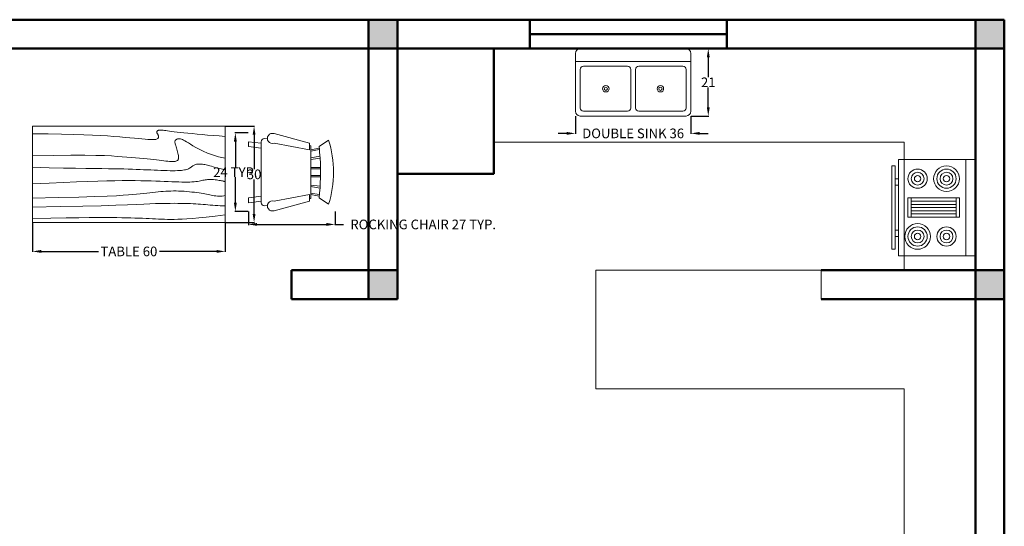
# Model space of a CAD drawing. Units: inches. Extents: x 13 to 1693, y -7 to 1519.
# Tile 4 of 10: x 377 to 683, y 577 to 735. Entities that reach past the tile are written whole.
import ezdxf

# ---------------------------------------------------------------- set-up
doc = ezdxf.new("R2010")
doc.units = ezdxf.units.IN
doc.header["$MEASUREMENT"] = 0
for name, color, linetype, lineweight in [('A-ANNO-DIMS', 2, 'Continuous', 18), ('A-FLOR-CASE', 5, 'Continuous', 18), ('A-FLOR-FIXT', 9, 'Continuous', 18), ('A-FURN', 8, 'Continuous', 18), ('A-WALL', 7, 'Continuous', 50), ('A-WALL-PATT', 8, 'Continuous', 13)]:
    doc.layers.add(name, color=color, linetype=linetype, lineweight=lineweight)
doc.styles.get("Standard").update_dxf_attribs({"font": 'arial.ttf'})
doc.dimstyles.get("Standard").update_dxf_attribs({"dimtxt": 3, "dimasz": 2.68, "dimexe": 0.18, "dimexo": 0.0625, "dimgap": 0.09, "dimtad": 0, "dimtih": 1, "dimtoh": 1, "dimdec": 0, "dimzin": 0, "dimdsep": 46, "dimlunit": 3, "dimtxsty": 'Standard', "dimcen": 0.09, "dimadec": 0, "dimazin": 0, "dimtfac": 1, "dimtdec": 0, "dimtofl": 0, "dimtmove": 0, "dimatfit": 3, "dimfxl": 1, "dimtolj": 1, "dimtzin": 0, "dimarcsym": 0})

# ---------------------------------------------------------------- blocks, each defined once
blk = doc.blocks.new('Chair - Rocking')
for p, q in [((-8, -4.5), (-10, -1.5)), ((8, -4.5), (10, -1.5)), ((-7.5, -4.5), (-7, -7)), ((-6.5, -7), (-7.02225, -4.43)), ((-4.5, -7), (-4.96674, -4.19951)), ((-4, -7), (-4.40532, -4.16272)), ((-1.5, -4.05012), (-1.5, -7)), ((-1, -7), (-1, -4.05012)), ((1, -7), (1, -4.04655)), ((1.5, -4.05012), (1.5, -7)), ((4, -7), (4.40187, -4.18694)), ((4.5, -7), (4.96761, -4.19437)), ((6.5, -7), (7, -4.4057)), ((7.5, -4.5), (7, -7)), ((-9, -7.5), (-12, -18.49999)), ((-7, -7.5), (-9, -7.5)), ((-9, -18.49999), (-7, -7.5)), ((-8.23428, -6.99939), (-8.3093, -7.47958)), ((-8.23041, -7), (8.23915, -7)), ((7, -7.5), (9, -7.5)), ((9, -18.49999), (7, -7.5)), ((8.31071, -7.48854), (8.23449, -7.00073)), ((9, -7.5), (12, -18.49999)), ((-10.36644, -20.64523), (-10.5, -21.49999)), ((10.5, -21.49999), (10.3575, -20.58798)), ((-9, -22.49999), (-9.5, -26.49999)), ((0, -22.49999), (-9.5, -22.49999)), ((-8, -26.49999), (-7.5, -22.49999)), ((0, -22.49999), (9.5, -22.49999)), ((8, -26.49999), (7.5, -22.49999)), ((9, -22.49999), (9.5, -26.49999)), ((-9.5, -26.49999), (-8, -26.49999)), ((9.5, -26.49999), (8, -26.49999))]:
    blk.add_line(p, q)
for centre, radius, start, end in [((0, -34.08333), 34.08333, 72.93847, 107.0615), ((0, -68.25004), 64.25, 93.92211, 97.15267), ((0, -68.25004), 64.25, 82.84733, 93.92211), ((-10.5, -18.99999), 1.58114, 161.5651, 18.43495), ((10.5, -18.99999), 1.58114, 161.5651, 18.43495), ((-9.5, -21.49999), 1, 180, 270), ((9.5, -21.49999), 1, 270, 0)]:
    blk.add_arc(centre, radius, start, end)
blk = doc.blocks.new('Table - Rectangular Woodgrain 60 x 30 in.')
for p, q in [((0, 0), (0, -30)), ((60, 0), (0, 0)), ((60, -30), (60, 0)), ((0, -30), (60, -30))]:
    blk.add_line(p, q)
for points in [[(0, -2.4), (4.8155, -2.418), (9.0302, -2.4688), (12.709, -2.5477), (15.9167, -2.65), (18.7181, -2.7711), (21.1781, -2.9063), (23.3616, -3.0508), (25.3333, -3.2), (27.1477, -3.3495), (28.8172, -3.4958), (30.3437, -3.636), (31.7291, -3.7667), (32.9756, -3.8849), (34.0849, -3.9875), (35.059, -4.0714), (35.9, -4.1334), (36.6114, -4.1711), (37.2041, -4.1854), (37.6906, -4.1779), (38.0833, -4.15), (38.3948, -4.1034), (38.6375, -4.0396), (38.8239, -3.9602), (38.9666, -3.8667), (39.0764, -3.7608), (39.1573, -3.6448), (39.2116, -3.521), (39.2416, -3.3917), (39.2498, -3.2593), (39.2385, -3.1261), (39.21, -2.9944), (39.1666, -2.8667), (39.111, -2.7447), (39.0468, -2.6281), (38.978, -2.5163), (38.9083, -2.4083), (38.8418, -2.3035), (38.7823, -2.201), (38.7337, -2.1001), (38.7, -2), (38.6844, -1.9003), (38.6875, -1.8021), (38.7094, -1.707), (38.75, -1.6167), (38.8094, -1.5326), (38.8875, -1.4563), (38.9844, -1.3893), (39.1, -1.3333), (39.2351, -1.2896), (39.3937, -1.2583), (39.5804, -1.2396), (39.8, -1.2333), (40.057, -1.2396), (40.3562, -1.2583), (40.7023, -1.2896), (41.1, -1.3333), (41.5547, -1.3895), (42.0755, -1.4573), (42.6721, -1.5361), (43.3542, -1.625), (44.1316, -1.7233), (45.014, -1.8302), (46.0114, -1.9449), (47.1333, -2.0667), (48.3862, -2.1947), (49.7625, -2.3281), (51.2513, -2.4663), (52.8416, -2.6083), (54.5226, -2.7535), (56.2833, -2.9011), (58.1127, -3.0501), (60, -3.2)], [(0, -9.2), (6.5759, -9.0858), (11.9385, -9.0365), (16.2527, -9.0418), (19.6833, -9.0917), (22.3952, -9.1759), (24.5531, -9.2844), (26.322, -9.4069), (27.8666, -9.5333), (29.3241, -9.6553), (30.7203, -9.7719), (32.0532, -9.8837), (33.3208, -9.9917), (34.5213, -10.0965), (35.6526, -10.199), (36.7128, -10.2999), (37.7, -10.4), (38.6129, -10.4996), (39.4531, -10.5969), (40.223, -10.6895), (40.925, -10.775), (41.5613, -10.8512), (42.1344, -10.9156), (42.6465, -10.966), (43.1, -11), (43.4976, -11.0158), (43.8437, -11.0136), (44.143, -10.9942), (44.4, -10.9583), (44.6195, -10.9069), (44.8062, -10.8406), (44.9648, -10.7603), (45.1, -10.6667), (45.2155, -10.5598), (45.3114, -10.4365), (45.3871, -10.2929), (45.4416, -10.125), (45.4743, -9.929), (45.4844, -9.7011), (45.4709, -9.4371), (45.4333, -9.1333), (45.3716, -8.7883), (45.2896, -8.4104), (45.1919, -8.0107), (45.0833, -7.6), (44.9685, -7.1893), (44.8521, -6.7896), (44.7388, -6.4117), (44.6333, -6.0667), (44.54, -5.7628), (44.4614, -5.4979), (44.4001, -5.2675), (44.3583, -5.0667), (44.3384, -4.8909), (44.3427, -4.7354), (44.3736, -4.5956), (44.4333, -4.4667), (44.5236, -4.3453), (44.6427, -4.2333), (44.7884, -4.1339), (44.9583, -4.05), (45.1501, -3.9849), (45.3614, -3.9417), (45.59, -3.9234), (45.8333, -3.9333), (46.0915, -3.9749), (46.3734, -4.0531), (46.6906, -4.1736), (47.0542, -4.3417), (47.4756, -4.5629), (47.9661, -4.8427), (48.5372, -5.1866), (49.2, -5.6), (49.9676, -6.0844), (50.8594, -6.625), (51.8965, -7.2031), (53.1, -7.8), (54.491, -8.3969), (56.0906, -8.975), (57.9199, -9.5156), (60, -10)], [(0, -12.8), (5.1847, -12.9322), (9.6213, -13.0323), (13.3963, -13.1059), (16.5958, -13.1583), (19.3063, -13.1952), (21.614, -13.2219), (23.6054, -13.2439), (25.3666, -13.2667), (26.9728, -13.2947), (28.4531, -13.3281), (29.8256, -13.3663), (31.1083, -13.4083), (32.3191, -13.4535), (33.476, -13.501), (34.597, -13.5501), (35.7, -13.6), (36.7984, -13.6497), (37.8875, -13.6979), (38.9578, -13.743), (40, -13.7833), (41.0047, -13.8174), (41.9625, -13.8438), (42.864, -13.8607), (43.7, -13.8667), (44.4631, -13.8604), (45.1552, -13.8417), (45.7801, -13.8104), (46.3416, -13.7667), (46.8439, -13.7104), (47.2906, -13.6417), (47.6858, -13.5604), (48.0333, -13.4667), (48.3375, -13.3608), (48.6042, -13.2448), (48.8396, -13.121), (49.05, -12.9917), (49.2417, -12.8593), (49.4208, -12.7261), (49.5937, -12.5944), (49.7667, -12.4667), (49.9452, -12.3451), (50.1323, -12.2313), (50.3303, -12.1268), (50.5416, -12.0333), (50.7686, -11.9524), (51.0135, -11.8854), (51.2788, -11.8341), (51.5666, -11.8), (51.8785, -11.7843), (52.2116, -11.7865), (52.562, -11.8059), (52.926, -11.8417), (53.2998, -11.8931), (53.6795, -11.9594), (54.0614, -12.0397), (54.4416, -12.1333), (54.8223, -12.2401), (55.2293, -12.3625), (55.6942, -12.5037), (56.2489, -12.6667), (56.9251, -12.8547), (57.7545, -13.0708), (58.7689, -13.3182), (60, -13.6)], [(0, -18), (5.124, -17.7273), (9.6609, -17.5057), (13.6705, -17.3303), (17.2125, -17.1958), (20.3467, -17.0973), (23.1328, -17.0297), (25.6307, -16.9878), (27.9, -16.9667), (29.9928, -16.9617), (31.9302, -16.9703), (33.7254, -16.9907), (35.3917, -17.0208), (36.9423, -17.0588), (38.3906, -17.1026), (39.7499, -17.1503), (41.0333, -17.2), (42.2519, -17.2496), (43.4073, -17.2969), (44.4986, -17.3395), (45.525, -17.375), (46.4858, -17.4012), (47.3802, -17.4156), (48.2074, -17.416), (48.9667, -17.4), (49.6583, -17.3662), (50.2872, -17.3167), (50.8595, -17.2547), (51.3812, -17.1833), (51.8584, -17.1057), (52.2971, -17.025), (52.7034, -16.9443), (53.0833, -16.8667), (53.443, -16.7951), (53.789, -16.7313), (54.128, -16.6768), (54.4666, -16.6334), (54.8115, -16.6024), (55.1693, -16.5854), (55.5465, -16.5841), (55.95, -16.6), (56.3828, -16.6337), (56.8346, -16.6823), (57.2915, -16.7418), (57.7396, -16.8084), (58.165, -16.878), (58.5539, -16.9469), (58.8924, -17.0111), (59.1666, -17.0667), (59.3679, -17.1107), (59.5078, -17.1438), (59.6032, -17.1675), (59.6708, -17.1833), (59.7275, -17.193), (59.7901, -17.1979), (59.8753, -17.1998), (60, -17.2)], [(0, -22.4), (8.0098, -22.2501), (14.4094, -22.1011), (19.4168, -21.9535), (23.25, -21.8083), (26.1269, -21.6663), (28.2656, -21.5281), (29.884, -21.3947), (31.2, -21.2667), (32.3967, -21.1448), (33.5172, -21.0292), (34.5697, -20.9198), (35.5625, -20.8167), (36.5037, -20.7198), (37.4015, -20.6292), (38.2642, -20.5448), (39.1, -20.4667), (39.9164, -20.3951), (40.7187, -20.3313), (41.5117, -20.2768), (42.3, -20.2333), (43.0883, -20.2024), (43.8812, -20.1854), (44.6836, -20.1841), (45.5, -20.2), (46.3328, -20.234), (47.1747, -20.2844), (48.0163, -20.3488), (48.8479, -20.425), (49.66, -20.5106), (50.4429, -20.6031), (51.1872, -20.7004), (51.8833, -20.8), (52.5246, -20.8999), (53.1166, -20.9995), (53.6681, -21.0983), (54.1875, -21.1958), (54.6834, -21.2919), (55.1646, -21.3859), (55.6394, -21.4777), (56.1167, -21.5667), (56.6028, -21.6515), (57.0961, -21.7266), (57.5929, -21.7852), (58.0896, -21.8208), (58.5823, -21.8268), (59.0674, -21.7964), (59.5412, -21.723), (60, -21.6)], [(0, -25.2), (8.6355, -25.0504), (15.7026, -24.9031), (21.4049, -24.7606), (25.9458, -24.625), (29.529, -24.4988), (32.3578, -24.3844), (34.6359, -24.284), (36.5667, -24.2), (38.3213, -24.1341), (39.9417, -24.0854), (41.437, -24.0523), (42.8167, -24.0333), (44.0901, -24.0268), (45.2667, -24.0313), (46.3557, -24.0451), (47.3667, -24.0667), (48.309, -24.0947), (49.1928, -24.1287), (50.0284, -24.168), (50.826, -24.2125), (51.5959, -24.2617), (52.3483, -24.3151), (53.0935, -24.3725), (53.8417, -24.4334), (54.6009, -24.497), (55.3699, -24.561), (56.1454, -24.6226), (56.9239, -24.6792), (57.7021, -24.7279), (58.4764, -24.7662), (59.2435, -24.7911), (60, -24.8)], [(0, -28.8), (5.6867, -28.6681), (10.45, -28.5698), (14.407, -28.5012), (17.675, -28.4584), (20.3711, -28.4374), (22.6125, -28.4344), (24.5164, -28.4455), (26.2, -28.4667), (27.762, -28.4947), (29.2276, -28.5281), (30.6033, -28.5663), (31.8958, -28.6084), (33.1118, -28.6535), (34.2578, -28.7011), (35.3405, -28.7501), (36.3666, -28.8), (37.3443, -28.8497), (38.288, -28.8974), (39.2137, -28.9412), (40.1375, -28.9792), (41.0753, -29.0093), (42.0432, -29.0297), (43.0572, -29.0384), (44.1333, -29.0333), (45.2936, -29.0114), (46.5843, -28.9641), (48.0579, -28.8816), (49.7666, -28.7542), (51.7629, -28.5721), (54.0989, -28.3255), (56.8272, -28.0048), (60, -27.6)]]:
    blk.add_lwpolyline(points)
blk = doc.blocks.new('Sink-double - 36 in top')
for p, q in [((-18, -4), (18, -4)), ((-0.75, -18.5), (-0.75, -6.5)), ((0.75, -6.5), (0.75, -18.5))]:
    blk.add_line(p, q)
for points in [[(-16.5, 0), (16.5, 0)], [(-18, -19.5), (-18, -1.5)], [(18, -1.5), (18, -19.5)], [(-15.5, -5.5), (-1.75, -5.5)], [(1.75, -5.5), (15.5, -5.5)], [(-16.5, -18.5), (-16.5, -6.5)], [(16.5, -6.5), (16.5, -18.5)], [(16.5, -21), (-16.5, -21)], [(-1.75, -19.5), (-15.5, -19.5)], [(15.5, -19.5), (1.75, -19.5)]]:
    blk.add_lwpolyline(points)
for centre, radius in [((-8.5, -12.5), 1), ((-8.5, -12.5), 0.5), ((8.5, -12.5), 1), ((8.5, -12.5), 0.5)]:
    blk.add_circle(centre, radius)
for centre, radius, start, end in [((-16.5, -1.5), 1.5, 90, 180), ((16.5, -1.5), 1.5, 0, 90), ((-15.5, -6.5), 1, 90, 180), ((-1.75, -6.5), 1, 0, 90), ((1.75, -6.5), 1, 90, 180), ((15.5, -6.5), 1, 0, 90), ((-16.5, -19.5), 1.5, 180, 270), ((-15.5, -18.5), 1, 180, 270), ((-1.75, -18.5), 1, 270, 0), ((1.75, -18.5), 1, 180, 270), ((15.5, -18.5), 1, 270, 0), ((16.5, -19.5), 1.5, 270, 0)]:
    blk.add_arc(centre, radius, start, end)
blk = doc.blocks.new('Range-Oven - 30 in top')
for p, q in [((0, -3), (30, -3)), ((12, -6), (18, -6)), ((13, -20), (13, -6)), ((14, -6), (14, -20)), ((15, -20), (15, -6)), ((16, -6), (16, -20)), ((17, -20), (17, -6)), ((18, -20), (12, -20)), ((6, -24), (6, -25)), ((8, -25), (8, -24)), ((22, -25), (22, -24)), ((24, -24), (24, -25))]:
    blk.add_line(p, q)
for points in [[(0, -24), (0, 0), (30, 0), (30, -24)], [(12, -21), (12, -5), (18, -5), (18, -21)], [(2, -26), (2, -25), (28, -25), (28, -26)]]:
    blk.add_lwpolyline(points, close=True)
for centre, radius in [((6, -9), 4), ((6, -9), 3), ((24, -9), 3), ((6, -9), 2), ((6, -9), 1), ((24, -9), 2), ((24, -9), 1), ((6, -18), 3), ((24, -18), 4), ((24, -18), 3), ((6, -18), 2), ((6, -18), 1), ((24, -18), 2), ((24, -18), 1)]:
    blk.add_circle(centre, radius)
blk = doc.blocks.new('*D56')
at = {"layer": 'A-ANNO-DIMS', "color": 0, "lineweight": -2, "transparency": 16777216}
for p, q in [((447.99, 675.39), (447.99, 671.22)), ((474.99, 675.39), (474.99, 671.22)), ((450.67, 671.4), (472.31, 671.4)), ((474.99, 671.4), (477.67, 671.4))]:
    blk.add_line(p, q, dxfattribs=at)
at = {"layer": 'A-ANNO-DIMS', "color": 0, "transparency": 16777216}
for points in [[(450.67, 671.85), (450.67, 670.96), (447.99, 671.4)], [(472.31, 671.85), (472.31, 670.96), (474.99, 671.4)]]:
    blk.add_solid(points, dxfattribs=at)
at = {"layer": 'Defpoints', "color": 0, "transparency": 16777216}
for p in [(447.99, 675.45), (474.99, 675.45), (474.99, 671.4)]:
    blk.add_point(p, dxfattribs=at)
at = {"layer": 'A-ANNO-DIMS', "color": 0, "transparency": 16777216, "insert": (502.44, 671.4), "char_height": 3, "attachment_point": 5}
blk.add_mtext('\\A1;ROCKING CHAIR 27 TYP.', dxfattribs=at)
blk = doc.blocks.new('*D57')
at = {"layer": 'A-ANNO-DIMS', "color": 0, "lineweight": -2, "transparency": 16777216}
for p, q in [((447.92, 699.89), (443.76, 699.89)), ((443.94, 697.21), (443.94, 689.27)), ((443.94, 678.13), (443.94, 686.07)), ((447.92, 675.45), (443.76, 675.45))]:
    blk.add_line(p, q, dxfattribs=at)
at = {"layer": 'A-ANNO-DIMS', "color": 0, "transparency": 16777216}
for points in [[(443.49, 697.21), (444.38, 697.21), (443.94, 699.89)], [(443.49, 678.13), (444.38, 678.13), (443.94, 675.45)]]:
    blk.add_solid(points, dxfattribs=at)
at = {"layer": 'Defpoints', "color": 0, "transparency": 16777216}
for p in [(447.99, 699.89), (443.94, 675.45), (447.99, 675.45)]:
    blk.add_point(p, dxfattribs=at)
at = {"layer": 'A-ANNO-DIMS', "color": 0, "transparency": 16777216, "insert": (443.94, 687.67), "char_height": 3, "attachment_point": 5}
blk.add_mtext('\\A1;24 TYP.', dxfattribs=at)
blk = doc.blocks.new('*D70')
at = {"layer": 'A-ANNO-DIMS', "color": 0, "lineweight": -2, "transparency": 16777216}
for p, q in [((380.77, 671.94), (380.77, 662.82)), ((440.77, 671.94), (440.77, 662.82)), ((383.45, 663), (401.28, 663)), ((438.09, 663), (420.26, 663))]:
    blk.add_line(p, q, dxfattribs=at)
at = {"layer": 'A-ANNO-DIMS', "color": 0, "transparency": 16777216}
for points in [[(383.45, 663.44), (383.45, 662.55), (380.77, 663)], [(438.09, 663.44), (438.09, 662.55), (440.77, 663)]]:
    blk.add_solid(points, dxfattribs=at)
at = {"layer": 'Defpoints', "color": 0, "transparency": 16777216}
for p in [(380.77, 672), (440.77, 672), (440.77, 663)]:
    blk.add_point(p, dxfattribs=at)
at = {"layer": 'A-ANNO-DIMS', "color": 0, "transparency": 16777216, "insert": (410.77, 663), "char_height": 3, "attachment_point": 5}
blk.add_mtext('\\A1;TABLE 60', dxfattribs=at)
blk = doc.blocks.new('*D71')
at = {"layer": 'A-ANNO-DIMS', "color": 0, "lineweight": -2, "transparency": 16777216}
for p, q in [((440.83, 702), (449.95, 702)), ((449.77, 699.32), (449.77, 688.62)), ((449.77, 674.68), (449.77, 685.38)), ((440.83, 672), (449.95, 672))]:
    blk.add_line(p, q, dxfattribs=at)
at = {"layer": 'A-ANNO-DIMS', "color": 0, "transparency": 16777216}
for points in [[(449.32, 699.32), (450.22, 699.32), (449.77, 702)], [(449.32, 674.68), (450.22, 674.68), (449.77, 672)]]:
    blk.add_solid(points, dxfattribs=at)
at = {"layer": 'Defpoints', "color": 0, "transparency": 16777216}
for p in [(440.77, 702), (449.77, 702), (440.77, 672)]:
    blk.add_point(p, dxfattribs=at)
at = {"layer": 'A-ANNO-DIMS', "color": 0, "transparency": 16777216, "insert": (449.77, 687), "char_height": 3, "attachment_point": 5}
blk.add_mtext('\\A1;30', dxfattribs=at)
blk = doc.blocks.new('*D72')
at = {"layer": 'A-ANNO-DIMS', "color": 0, "lineweight": -2, "transparency": 16777216}
for p, q in [((549.84, 705.09), (549.84, 699.57)), ((585.84, 705.09), (585.84, 699.57)), ((547.16, 699.75), (544.48, 699.75)), ((588.52, 699.75), (591.2, 699.75))]:
    blk.add_line(p, q, dxfattribs=at)
at = {"layer": 'A-ANNO-DIMS', "color": 0, "transparency": 16777216}
for points in [[(547.16, 700.2), (547.16, 699.3), (549.84, 699.75)], [(588.52, 700.2), (588.52, 699.3), (585.84, 699.75)]]:
    blk.add_solid(points, dxfattribs=at)
at = {"layer": 'Defpoints', "color": 0, "transparency": 16777216}
for p in [(549.84, 705.15), (585.84, 705.15), (585.84, 699.75)]:
    blk.add_point(p, dxfattribs=at)
at = {"layer": 'A-ANNO-DIMS', "color": 0, "transparency": 16777216, "insert": (567.84, 699.75), "char_height": 3, "attachment_point": 5}
blk.add_mtext('\\A1;DOUBLE SINK 36', dxfattribs=at)
blk = doc.blocks.new('*D73')
at = {"layer": 'A-ANNO-DIMS', "color": 0, "lineweight": -2, "transparency": 16777216}
for p, q in [((585.91, 726.15), (591.42, 726.15)), ((591.24, 723.47), (591.24, 717.25)), ((591.24, 707.83), (591.24, 714.05)), ((585.91, 705.15), (591.42, 705.15))]:
    blk.add_line(p, q, dxfattribs=at)
at = {"layer": 'A-ANNO-DIMS', "color": 0, "transparency": 16777216}
for points in [[(590.8, 723.47), (591.69, 723.47), (591.24, 726.15)], [(590.8, 707.83), (591.69, 707.83), (591.24, 705.15)]]:
    blk.add_solid(points, dxfattribs=at)
at = {"layer": 'Defpoints', "color": 0, "transparency": 16777216}
for p in [(585.84, 726.15), (591.24, 726.15), (585.84, 705.15)]:
    blk.add_point(p, dxfattribs=at)
at = {"layer": 'A-ANNO-DIMS', "color": 0, "transparency": 16777216, "insert": (591.24, 715.65), "char_height": 3, "attachment_point": 5}
blk.add_mtext('\\A1;21', dxfattribs=at)

msp = doc.modelspace()

# ---------------------------------------------------------------- hatches: boundary and pattern name
at = {"layer": 'A-WALL-PATT'}
h = msp.add_hatch(color=256, dxfattribs=at)
h.dxf.hatch_style = 1
h.paths.add_polyline_path([(494.45, 657.15), (485.45, 657.15), (485.45, 648.15), (494.45, 648.15)])
h.paths.add_polyline_path([(494.45, 735.15), (485.45, 735.15), (485.45, 726.15), (494.45, 726.15)])
h = msp.add_hatch(color=256, dxfattribs=at)
h.dxf.hatch_style = 1
h.paths.add_polyline_path([(683.45, 735.15), (674.45, 735.15), (674.45, 726.15), (683.45, 726.15)])
h.paths.add_polyline_path([(683.45, 657.15), (674.45, 657.15), (674.45, 648.15), (683.45, 648.15)])
h.paths.add_polyline_path([(494.45, 498.15), (485.45, 498.15), (485.45, 489.15), (494.45, 489.15)])
h.paths.add_polyline_path([(683.45, 498.15), (674.45, 498.15), (674.45, 489.15), (683.45, 489.15)])
h.paths.add_polyline_path([(494.45, 222.15), (485.45, 222.15), (485.45, 213.15), (494.45, 213.15)])
h.paths.add_polyline_path([(683.45, 369.15), (674.45, 369.15), (674.45, 360.15), (683.45, 360.15)])

# ---------------------------------------------------------------- linework, layer by layer
at = {"layer": 'A-FLOR-CASE'}
for p, q in [((524.42, 696.99), (652.22, 696.99)), ((652.22, 696.99), (652.22, 657.15)), ((652.22, 657.15), (556.27, 657.15)), ((556.27, 657.15), (556.27, 620.17)), ((626.45, 648.15), (626.45, 657.15)), ((650.45, 648.15), (626.45, 648.15)), ((556.27, 620.17), (652.22, 620.17)), ((652.22, 620.17), (652.22, 522.4))]:
    msp.add_line(p, q, dxfattribs=at)
at = {"layer": 'A-WALL'}
for p, q in [((683.45, 735.15), (116.45, 735.15)), ((485.45, 648.15), (485.45, 735.15)), ((494.45, 648.15), (494.45, 735.15)), ((535.69, 735.15), (535.69, 726.15)), ((597.02, 735.15), (597.02, 726.15)), ((683.45, 147.15), (683.45, 735.15)), ((535.69, 730.65), (597.02, 730.65)), ((485.45, 726.15), (116.45, 726.15)), ((674.45, 726.15), (494.45, 726.15)), ((674.45, 657.15), (674.45, 726.15)), ((494.45, 657.15), (461.45, 657.15)), ((461.45, 648.15), (461.45, 657.15)), ((674.45, 657.15), (626.45, 657.15)), ((494.45, 648.15), (461.45, 648.15)), ((674.45, 648.15), (626.45, 648.15)), ((674.45, 498.15), (674.45, 648.15))]:
    msp.add_line(p, q, dxfattribs=at)
for points in [[(485.45, 726.15), (494.45, 726.15), (494.45, 735.15), (485.45, 735.15)], [(683.45, 735.15), (674.45, 735.15), (674.45, 726.15), (683.45, 726.15)], [(494.45, 726.15), (524.42, 726.15), (524.42, 687.19), (494.45, 687.19)], [(674.45, 657.15), (683.45, 657.15), (683.45, 648.15), (674.45, 648.15)]]:
    msp.add_lwpolyline(points, close=True, dxfattribs=at)

# ---------------------------------------------------------------- block references
at = {"layer": 'A-FLOR-FIXT'}
msp.add_blockref('Sink-double - 36 in top', (567.84, 726.15), dxfattribs=at)
at = {"layer": 'A-FLOR-FIXT', "rotation": 270}
msp.add_blockref('Range-Oven - 30 in top', (674.45, 691.65), dxfattribs=at)
at = {"layer": 'A-FURN'}
msp.add_blockref('Table - Rectangular Woodgrain 60 x 30 in.', (380.77, 702), dxfattribs=at)
at = {"layer": 'A-FURN', "rotation": 270}
msp.add_blockref('Chair - Rocking', (474.49, 687.67), dxfattribs=at)

# ---------------------------------------------------------------- dimensions: what is measured, and where the dimension line sits
at = {"layer": 'A-ANNO-DIMS'}
for base, p1, p2, picture, middle in [((591.24, 726.15), (585.84, 705.15), (585.84, 726.15), '*D73', (591.24, 715.65)), ((449.77, 702), (440.77, 672), (440.77, 702), '*D71', (449.77, 687))]:
    dim = msp.add_linear_dim(base=base, p1=p1, p2=p2, angle=90, dimstyle='Standard', override={"dimdec": 0, "dimlfac": 1, "dimrnd": 0, "dimzin": 0, "dimdsep": 46, "dimlunit": 2}, dxfattribs=at)
    dim.commit()
    dim.dimension.update_dxf_attribs({"geometry": picture, "text_midpoint": middle})
for base, p1, p2, text, picture, middle in [((585.84, 699.75), (549.84, 705.15), (585.84, 705.15), 'DOUBLE SINK <>', '*D72', (567.84, 699.75)), ((474.99, 671.4), (447.99, 675.45), (474.99, 675.45), 'ROCKING CHAIR <> TYP.', '*D56', (502.44, 671.4)), ((440.77, 663), (380.77, 672), (440.77, 672), 'TABLE <>', '*D70', (410.77, 663))]:
    dim = msp.add_linear_dim(base=base, p1=p1, p2=p2, text=text, dimstyle='Standard', override={"dimdec": 0, "dimlfac": 1, "dimrnd": 0, "dimzin": 0, "dimdsep": 46, "dimlunit": 2}, dxfattribs=at)
    dim.commit()
    dim.dimension.update_dxf_attribs({"geometry": picture, "text_midpoint": middle})
dim = msp.add_linear_dim(base=(443.94, 675.45), p1=(447.99, 699.89), p2=(447.99, 675.45), angle=270, text='<> TYP.', dimstyle='Standard', override={"dimdec": 0, "dimlfac": 1, "dimrnd": 0, "dimzin": 0, "dimdsep": 46, "dimlunit": 2}, dxfattribs=at)
dim.commit()
dim.dimension.update_dxf_attribs({"geometry": '*D57', "text_midpoint": (443.94, 687.67)})

doc.saveas('drawing.dxf')
